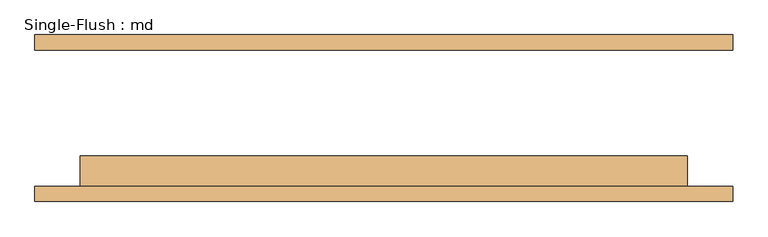
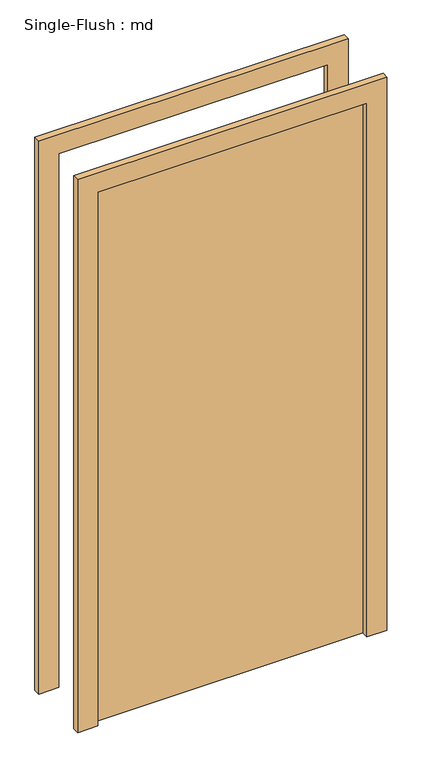
"""IFC4 building model written with IfcOpenShell, lengths in millimetres: door geometry, Single-Flush : md."""

from ifc_helpers import new_model, si_unit, frame, origin, origin_with_axes, place, context, project, spatial, polyline, outline, extrude, source, transform, mapped, element, save


def single_flush_md_8244dad1(model_context):
    return source(origin(), model_context, "Body", "SweptSolid", [
        extrude(outline(polyline([(2209.8, -584.2), (0.0, -584.2), (0.0, -508.0), (2133.6, -508.0), (2133.6, 508.0), (0.0, 508.0), (0.0, 584.2), (2209.8, 584.2), (2209.8, -584.2)])), frame((0.0, -139.7, 0.0), z_axis=(0.0, 1.0, 0.0), x_axis=(0.0, 0.0, 1.0)), (0.0, 0.0, 1.0), 25.4),
        extrude(outline(polyline([(2209.8, 584.2), (2209.8, -584.2), (0.0, -584.2), (0.0, -508.0), (2133.6, -508.0), (2133.6, 508.0), (0.0, 508.0), (0.0, 584.2), (2209.8, 584.2)])), frame((0.0, 114.3, 0.0), z_axis=(0.0, 1.0, 0.0), x_axis=(0.0, 0.0, 1.0)), (0.0, 0.0, 1.0), 25.4),
        extrude(outline(polyline([(508.0, -63.5), (508.0, -114.3), (-508.0, -114.3), (-508.0, -63.5), (508.0, -63.5)])), origin_with_axes(), (0.0, 0.0, 1.0), 2133.6),
    ])


if __name__ == "__main__":
    model = new_model("IFC4")
    model_context = context("Model", 3, world=origin())
    ifc_project = project(units=[si_unit("LENGTHUNIT", "METRE", prefix="MILLI")], contexts=[model_context])
    site = spatial("IfcSite", under=ifc_project)
    building = spatial("IfcBuilding", under=site)
    placement = place(None, origin())
    single_flush_md_shape = single_flush_md_8244dad1(model_context)
    element("IfcDoor", 1, ObjectType="Single-Flush : md", at=placement, inside=building, context=model_context, shape_type="MappedRepresentation", body=[
        mapped(single_flush_md_shape, transform((0.0, 0.0, 0.0), x_axis=(1.0, 0.0, 0.0), y_axis=(0.0, 1.0, 0.0), z_axis=(0.0, 0.0, 1.0))),
    ])
    save(model, "model.ifc")

# Revit data of these elements
# Type "Single-Flush : md"
#   Type Mark = "8"
#   Construction Type Id = "MDOOR"
#   Assembly Code = "C1020"
#   Analytic Construction = "Metal"
#   Thickness = 0' - 2"
#   Heat Transfer Coefficient (U) = 0.651978 BTU/(h·ft²·°F)
#   Height = 7' - 0"
#   Trim Projection Ext = 0' - 1"
#   Trim Projection Int = 0' - 1"
#   Trim Width = 0' - 3"
#   Width = 3' - 4"
#   Define Thermal Properties by = 1
#   Door Material = Door - Panel
#   Frame Material = Door - Frame
#   Visual Light Transmittance = 0
#   Solar Heat Gain Coefficient = 0
#   Function = (empty or 0)
#   Wall Closure = (empty or 0)
# Element 1 (IfcDoor, "Single-Flush : md")
#   Materials on its faces: "Door - Frame", "Door - Panel"
# Materials
#   "Door - Panel": class "Wood", colour RGB 210 159 95, transparency 0, Cost = 0
#   "Door - Frame": colour RGB 118 70 51, transparency 0, Cost = 0
